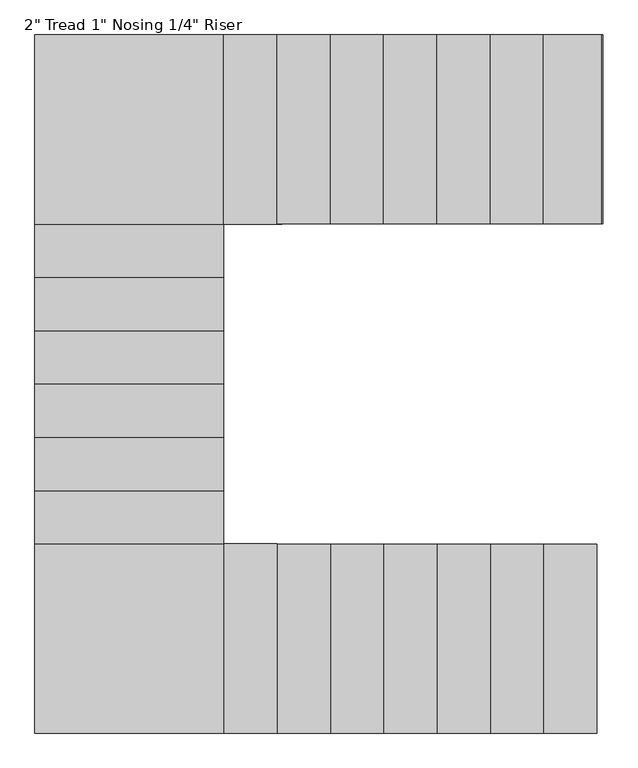
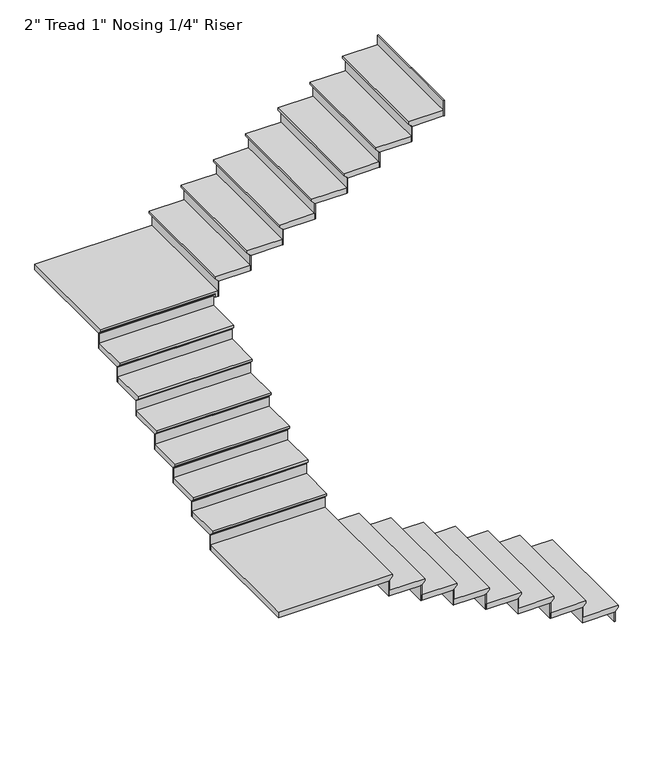
"""IFC4 building model written with IfcOpenShell, lengths in millimetres: stair flight geometry."""

from ifc_helpers import new_model, si_unit, origin, place, context, project, spatial, faceted_brep, source, transform, mapped, element, save


def stair_flight_046a0556(model_context):
    return source(origin(), model_context, "Body", "Brep", [
        faceted_brep([(-1428.1308482, -127.8399287, 119.4954545), (-1428.1308482, -127.8399287, 138.5454545), (-1428.1308482, -1118.4399287, 138.5454545), (-1428.1308482, -1118.4399287, 119.4954545), (-1453.5308482, -127.8399287, 94.0954545), (-1453.5308482, -1118.4399287, 94.0954545), (-1732.9308482, -127.8399287, 138.5454545), (-1732.9308482, -1118.4399287, 138.5454545), (-1453.5308482, -1118.4399287, 87.7454545), (-1732.9308482, -1118.4399287, 87.7454545), (-1732.9308482, -127.8399287, 87.7454545), (-1453.5308482, -127.8399287, 87.7454545)], [[[0, 1, 2, 3]], [[4, 0, 3, 5]], [[2, 1, 6, 7]], [[8, 9, 10, 11]], [[2, 7, 9, 8, 5, 3]], [[8, 11, 4, 5]], [[6, 1, 0, 4, 11, 10]], [[7, 6, 10, 9]]]),
        faceted_brep([(-1453.5308482, -127.8399287, 87.7454545), (-1453.5308482, -127.8399287, 0.0), (-1459.8808482, -127.8399287, 0.0), (-1459.8808482, -127.8399287, 87.7454545), (-1453.5308482, -1118.4399287, 87.7454545), (-1459.8808482, -1118.4399287, 87.7454545), (-1459.8808482, -1118.4399287, 0.0), (-1453.5308482, -1118.4399287, 0.0)], [[[0, 1, 2, 3]], [[4, 5, 6, 7]], [[1, 0, 4, 7]], [[2, 1, 7, 6]], [[3, 2, 6, 5]], [[0, 3, 5, 4]]]),
        faceted_brep([(-1732.9308482, -127.8399287, 226.2909091), (-1732.9308482, -127.8399287, 87.7454545), (-1739.2808482, -127.8399287, 87.7454545), (-1739.2808482, -127.8399287, 226.2909091), (-1732.9308482, -1118.4399287, 226.2909091), (-1739.2808482, -1118.4399287, 226.2909091), (-1739.2808482, -1118.4399287, 87.7454545), (-1732.9308482, -1118.4399287, 87.7454545)], [[[0, 1, 2, 3]], [[4, 5, 6, 7]], [[1, 0, 4, 7]], [[2, 1, 7, 6]], [[3, 2, 6, 5]], [[0, 3, 5, 4]]]),
        faceted_brep([(-1707.5308482, -1118.4399287, 277.0909091), (-1707.5308482, -127.8399287, 277.0909091), (-2012.3308482, -127.8399287, 277.0909091), (-2012.3308482, -1118.4399287, 277.0909091), (-1732.9308482, -1118.4399287, 226.2909091), (-2012.3308482, -1118.4399287, 226.2909091), (-2012.3308482, -127.8399287, 226.2909091), (-1732.9308482, -127.8399287, 226.2909091), (-1732.9308482, -1118.4399287, 232.6409091), (-1707.5308482, -1118.4399287, 258.0409091), (-1732.9308482, -127.8399287, 232.6409091), (-1707.5308482, -127.8399287, 258.0409091)], [[[0, 1, 2, 3]], [[4, 5, 6, 7]], [[0, 3, 5, 4, 8, 9]], [[4, 7, 10, 8]], [[2, 1, 11, 10, 7, 6]], [[3, 2, 6, 5]], [[11, 1, 0, 9]], [[10, 11, 9, 8]]]),
        faceted_brep([(-2012.3308482, -127.8399287, 364.8363636), (-2012.3308482, -127.8399287, 226.2909091), (-2018.6808482, -127.8399287, 226.2909091), (-2018.6808482, -127.8399287, 364.8363636), (-2012.3308482, -1118.4399287, 364.8363636), (-2018.6808482, -1118.4399287, 364.8363636), (-2018.6808482, -1118.4399287, 226.2909091), (-2012.3308482, -1118.4399287, 226.2909091)], [[[0, 1, 2, 3]], [[4, 5, 6, 7]], [[1, 0, 4, 7]], [[2, 1, 7, 6]], [[3, 2, 6, 5]], [[0, 3, 5, 4]]]),
        faceted_brep([(-1986.9308482, -1118.4399287, 415.6363636), (-1986.9308482, -127.8399287, 415.6363636), (-2291.7308482, -127.8399287, 415.6363636), (-2291.7308482, -1118.4399287, 415.6363636), (-2012.3308482, -1118.4399287, 364.8363636), (-2291.7308482, -1118.4399287, 364.8363636), (-2291.7308482, -127.8399287, 364.8363636), (-2012.3308482, -127.8399287, 364.8363636), (-2012.3308482, -1118.4399287, 371.1863636), (-1986.9308482, -1118.4399287, 396.5863636), (-2012.3308482, -127.8399287, 371.1863636), (-1986.9308482, -127.8399287, 396.5863636)], [[[0, 1, 2, 3]], [[4, 5, 6, 7]], [[0, 3, 5, 4, 8, 9]], [[4, 7, 10, 8]], [[2, 1, 11, 10, 7, 6]], [[3, 2, 6, 5]], [[11, 1, 0, 9]], [[10, 11, 9, 8]]]),
        faceted_brep([(-2291.7308482, -127.8399287, 503.3818182), (-2291.7308482, -127.8399287, 364.8363636), (-2298.0808482, -127.8399287, 364.8363636), (-2298.0808482, -127.8399287, 503.3818182), (-2291.7308482, -1118.4399287, 503.3818182), (-2298.0808482, -1118.4399287, 503.3818182), (-2298.0808482, -1118.4399287, 364.8363636), (-2291.7308482, -1118.4399287, 364.8363636)], [[[0, 1, 2, 3]], [[4, 5, 6, 7]], [[1, 0, 4, 7]], [[2, 1, 7, 6]], [[3, 2, 6, 5]], [[0, 3, 5, 4]]]),
        faceted_brep([(-2266.3308482, -1118.4399287, 554.1818182), (-2266.3308482, -127.8399287, 554.1818182), (-2571.1308482, -127.8399287, 554.1818182), (-2571.1308482, -1118.4399287, 554.1818182), (-2291.7308482, -1118.4399287, 503.3818182), (-2571.1308482, -1118.4399287, 503.3818182), (-2571.1308482, -127.8399287, 503.3818182), (-2291.7308482, -127.8399287, 503.3818182), (-2291.7308482, -1118.4399287, 509.7318182), (-2266.3308482, -1118.4399287, 535.1318182), (-2291.7308482, -127.8399287, 509.7318182), (-2266.3308482, -127.8399287, 535.1318182)], [[[0, 1, 2, 3]], [[4, 5, 6, 7]], [[0, 3, 5, 4, 8, 9]], [[4, 7, 10, 8]], [[2, 1, 11, 10, 7, 6]], [[3, 2, 6, 5]], [[11, 1, 0, 9]], [[10, 11, 9, 8]]]),
        faceted_brep([(-2571.1308482, -127.8399287, 641.9272727), (-2571.1308482, -127.8399287, 503.3818182), (-2577.4808482, -127.8399287, 503.3818182), (-2577.4808482, -127.8399287, 641.9272727), (-2571.1308482, -1118.4399287, 641.9272727), (-2577.4808482, -1118.4399287, 641.9272727), (-2577.4808482, -1118.4399287, 503.3818182), (-2571.1308482, -1118.4399287, 503.3818182)], [[[0, 1, 2, 3]], [[4, 5, 6, 7]], [[1, 0, 4, 7]], [[2, 1, 7, 6]], [[3, 2, 6, 5]], [[0, 3, 5, 4]]]),
        faceted_brep([(-2545.7308482, -1118.4399287, 692.7272727), (-2545.7308482, -127.8399287, 692.7272727), (-2850.5308482, -127.8399287, 692.7272727), (-2850.5308482, -1118.4399287, 692.7272727), (-2571.1308482, -1118.4399287, 641.9272727), (-2850.5308482, -1118.4399287, 641.9272727), (-2850.5308482, -127.8399287, 641.9272727), (-2571.1308482, -127.8399287, 641.9272727), (-2571.1308482, -1118.4399287, 648.2772727), (-2545.7308482, -1118.4399287, 673.6772727), (-2571.1308482, -127.8399287, 648.2772727), (-2545.7308482, -127.8399287, 673.6772727)], [[[0, 1, 2, 3]], [[4, 5, 6, 7]], [[0, 3, 5, 4, 8, 9]], [[4, 7, 10, 8]], [[2, 1, 11, 10, 7, 6]], [[3, 2, 6, 5]], [[11, 1, 0, 9]], [[10, 11, 9, 8]]]),
        faceted_brep([(-2850.5308482, -127.8399287, 780.4727273), (-2850.5308482, -127.8399287, 641.9272727), (-2856.8808482, -127.8399287, 641.9272727), (-2856.8808482, -127.8399287, 780.4727273), (-2850.5308482, -1118.4399287, 780.4727273), (-2856.8808482, -1118.4399287, 780.4727273), (-2856.8808482, -1118.4399287, 641.9272727), (-2850.5308482, -1118.4399287, 641.9272727)], [[[0, 1, 2, 3]], [[4, 5, 6, 7]], [[1, 0, 4, 7]], [[2, 1, 7, 6]], [[3, 2, 6, 5]], [[0, 3, 5, 4]]]),
        faceted_brep([(-2825.1308482, -1118.4399287, 831.2727273), (-2825.1308482, -127.8399287, 831.2727273), (-3129.9308482, -127.8399287, 831.2727273), (-3129.9308482, -1118.4399287, 831.2727273), (-2850.5308482, -1118.4399287, 780.4727273), (-3129.9308482, -1118.4399287, 780.4727273), (-3129.9308482, -127.8399287, 780.4727273), (-2850.5308482, -127.8399287, 780.4727273), (-2850.5308482, -1118.4399287, 786.8227273), (-2825.1308482, -1118.4399287, 812.2227273), (-2850.5308482, -127.8399287, 786.8227273), (-2825.1308482, -127.8399287, 812.2227273)], [[[0, 1, 2, 3]], [[4, 5, 6, 7]], [[0, 3, 5, 4, 8, 9]], [[4, 7, 10, 8]], [[2, 1, 11, 10, 7, 6]], [[3, 2, 6, 5]], [[11, 1, 0, 9]], [[10, 11, 9, 8]]]),
        faceted_brep([(-3129.9308482, -127.8399287, 919.0181818), (-3129.9308482, -127.8399287, 780.4727273), (-3136.2808482, -127.8399287, 780.4727273), (-3136.2808482, -127.8399287, 919.0181818), (-3129.9308482, -1118.4399287, 919.0181818), (-3136.2808482, -1118.4399287, 919.0181818), (-3136.2808482, -1118.4399287, 780.4727273), (-3129.9308482, -1118.4399287, 780.4727273)], [[[0, 1, 2, 3]], [[4, 5, 6, 7]], [[1, 0, 4, 7]], [[2, 1, 7, 6]], [[3, 2, 6, 5]], [[0, 3, 5, 4]]]),
        faceted_brep([(-3104.5308482, -1118.4399287, 969.8181818), (-3104.5308482, -127.8399287, 969.8181818), (-3409.3308482, -127.8399287, 969.8181818), (-3409.3308482, -1118.4399287, 969.8181818), (-3129.9308482, -1118.4399287, 919.0181818), (-3409.3308482, -1118.4399287, 919.0181818), (-3409.3308482, -127.8399287, 919.0181818), (-3129.9308482, -127.8399287, 919.0181818), (-3129.9308482, -1118.4399287, 925.3681818), (-3104.5308482, -1118.4399287, 950.7681818), (-3129.9308482, -127.8399287, 925.3681818), (-3104.5308482, -127.8399287, 950.7681818)], [[[0, 1, 2, 3]], [[4, 5, 6, 7]], [[0, 3, 5, 4, 8, 9]], [[4, 7, 10, 8]], [[2, 1, 11, 10, 7, 6]], [[3, 2, 6, 5]], [[11, 1, 0, 9]], [[10, 11, 9, 8]]]),
        faceted_brep([(-3409.3308482, -127.8399287, 1057.5636364), (-3409.3308482, -127.8399287, 919.0181818), (-3415.6808482, -127.8399287, 919.0181818), (-3415.6808482, -127.8399287, 1057.5636364), (-3409.3308482, -1118.4399287, 1057.5636364), (-3415.6808482, -1118.4399287, 1057.5636364), (-3415.6808482, -1118.4399287, 919.0181818), (-3409.3308482, -1118.4399287, 919.0181818)], [[[0, 1, 2, 3]], [[4, 5, 6, 7]], [[1, 0, 4, 7]], [[2, 1, 7, 6]], [[3, 2, 6, 5]], [[0, 3, 5, 4]]]),
        faceted_brep([(-4374.5308482, -102.4399287, 1108.3636364), (-4374.5308482, -1118.4399287, 1108.3636364), (-3383.9308482, -1118.4399287, 1108.3636364), (-3383.9308482, -102.4399287, 1108.3636364), (-4374.5308482, -1118.4399287, 1057.5636364), (-4374.5308482, -102.4399287, 1057.5636364), (-3383.9308482, -102.4399287, 1057.5636364), (-3383.9308482, -127.8399287, 1057.5636364), (-3409.3308482, -127.8399287, 1057.5636364), (-3409.3308482, -1118.4399287, 1057.5636364), (-3409.3308482, -127.8399287, 1063.9136364), (-3409.3308482, -1118.4399287, 1063.9136364), (-3383.9308482, -1118.4399287, 1089.3136364), (-3383.9308482, -127.8399287, 1089.3136364)], [[[0, 1, 2, 3]], [[4, 5, 6, 7, 8, 9]], [[1, 0, 5, 4]], [[9, 8, 10, 11]], [[3, 2, 12, 13, 7, 6]], [[0, 3, 6, 5]], [[12, 11, 10, 13]], [[2, 1, 4, 9, 11, 12]], [[8, 7, 13, 10]]]),
        faceted_brep([(-3383.9308482, -102.4399287, 1196.1090909), (-3383.9308482, -102.4399287, 1057.5636364), (-3383.9308482, -96.0899287, 1057.5636364), (-3383.9308482, -96.0899287, 1196.1090909), (-4374.5308482, -102.4399287, 1196.1090909), (-4374.5308482, -96.0899287, 1196.1090909), (-4374.5308482, -96.0899287, 1057.5636364), (-4374.5308482, -102.4399287, 1057.5636364)], [[[0, 1, 2, 3]], [[4, 5, 6, 7]], [[1, 0, 4, 7]], [[2, 1, 7, 6]], [[3, 2, 6, 5]], [[0, 3, 5, 4]]]),
        faceted_brep([(-4374.5308482, -127.8399287, 1246.9090909), (-3383.9308482, -127.8399287, 1246.9090909), (-3383.9308482, 176.9600713, 1246.9090909), (-4374.5308482, 176.9600713, 1246.9090909), (-4374.5308482, -102.4399287, 1196.1090909), (-4374.5308482, 176.9600713, 1196.1090909), (-3383.9308482, 176.9600713, 1196.1090909), (-3383.9308482, -102.4399287, 1196.1090909), (-4374.5308482, -102.4399287, 1202.4590909), (-4374.5308482, -127.8399287, 1227.8590909), (-3383.9308482, -102.4399287, 1202.4590909), (-3383.9308482, -127.8399287, 1227.8590909)], [[[0, 1, 2, 3]], [[4, 5, 6, 7]], [[0, 3, 5, 4, 8, 9]], [[4, 7, 10, 8]], [[2, 1, 11, 10, 7, 6]], [[3, 2, 6, 5]], [[11, 1, 0, 9]], [[10, 11, 9, 8]]]),
        faceted_brep([(-3383.9308482, 176.9600713, 1334.6545455), (-3383.9308482, 176.9600713, 1196.1090909), (-3383.9308482, 183.3100713, 1196.1090909), (-3383.9308482, 183.3100713, 1334.6545455), (-4374.5308482, 176.9600713, 1334.6545455), (-4374.5308482, 183.3100713, 1334.6545455), (-4374.5308482, 183.3100713, 1196.1090909), (-4374.5308482, 176.9600713, 1196.1090909)], [[[0, 1, 2, 3]], [[4, 5, 6, 7]], [[1, 0, 4, 7]], [[2, 1, 7, 6]], [[3, 2, 6, 5]], [[0, 3, 5, 4]]]),
        faceted_brep([(-4374.5308482, 151.5600713, 1385.4545455), (-3383.9308482, 151.5600713, 1385.4545455), (-3383.9308482, 456.3600713, 1385.4545455), (-4374.5308482, 456.3600713, 1385.4545455), (-4374.5308482, 176.9600713, 1334.6545455), (-4374.5308482, 456.3600713, 1334.6545455), (-3383.9308482, 456.3600713, 1334.6545455), (-3383.9308482, 176.9600713, 1334.6545455), (-4374.5308482, 176.9600713, 1341.0045455), (-4374.5308482, 151.5600713, 1366.4045455), (-3383.9308482, 176.9600713, 1341.0045455), (-3383.9308482, 151.5600713, 1366.4045455)], [[[0, 1, 2, 3]], [[4, 5, 6, 7]], [[0, 3, 5, 4, 8, 9]], [[4, 7, 10, 8]], [[2, 1, 11, 10, 7, 6]], [[3, 2, 6, 5]], [[11, 1, 0, 9]], [[10, 11, 9, 8]]]),
        faceted_brep([(-3383.9308482, 456.3600713, 1473.2), (-3383.9308482, 456.3600713, 1334.6545455), (-3383.9308482, 462.7100713, 1334.6545455), (-3383.9308482, 462.7100713, 1473.2), (-4374.5308482, 456.3600713, 1473.2), (-4374.5308482, 462.7100713, 1473.2), (-4374.5308482, 462.7100713, 1334.6545455), (-4374.5308482, 456.3600713, 1334.6545455)], [[[0, 1, 2, 3]], [[4, 5, 6, 7]], [[1, 0, 4, 7]], [[2, 1, 7, 6]], [[3, 2, 6, 5]], [[0, 3, 5, 4]]]),
        faceted_brep([(-4374.5308482, 430.9600713, 1524.0), (-3383.9308482, 430.9600713, 1524.0), (-3383.9308482, 735.7600713, 1524.0), (-4374.5308482, 735.7600713, 1524.0), (-4374.5308482, 456.3600713, 1473.2), (-4374.5308482, 735.7600713, 1473.2), (-3383.9308482, 735.7600713, 1473.2), (-3383.9308482, 456.3600713, 1473.2), (-4374.5308482, 456.3600713, 1479.55), (-4374.5308482, 430.9600713, 1504.95), (-3383.9308482, 456.3600713, 1479.55), (-3383.9308482, 430.9600713, 1504.95)], [[[0, 1, 2, 3]], [[4, 5, 6, 7]], [[0, 3, 5, 4, 8, 9]], [[4, 7, 10, 8]], [[2, 1, 11, 10, 7, 6]], [[3, 2, 6, 5]], [[11, 1, 0, 9]], [[10, 11, 9, 8]]]),
        faceted_brep([(-3383.9308482, 735.7600713, 1611.7454545), (-3383.9308482, 735.7600713, 1473.2), (-3383.9308482, 742.1100713, 1473.2), (-3383.9308482, 742.1100713, 1611.7454545), (-4374.5308482, 735.7600713, 1611.7454545), (-4374.5308482, 742.1100713, 1611.7454545), (-4374.5308482, 742.1100713, 1473.2), (-4374.5308482, 735.7600713, 1473.2)], [[[0, 1, 2, 3]], [[4, 5, 6, 7]], [[1, 0, 4, 7]], [[2, 1, 7, 6]], [[3, 2, 6, 5]], [[0, 3, 5, 4]]]),
        faceted_brep([(-4374.5308482, 710.3600713, 1662.5454545), (-3383.9308482, 710.3600713, 1662.5454545), (-3383.9308482, 1015.1600713, 1662.5454545), (-4374.5308482, 1015.1600713, 1662.5454545), (-4374.5308482, 735.7600713, 1611.7454545), (-4374.5308482, 1015.1600713, 1611.7454545), (-3383.9308482, 1015.1600713, 1611.7454545), (-3383.9308482, 735.7600713, 1611.7454545), (-4374.5308482, 735.7600713, 1618.0954545), (-4374.5308482, 710.3600713, 1643.4954545), (-3383.9308482, 735.7600713, 1618.0954545), (-3383.9308482, 710.3600713, 1643.4954545)], [[[0, 1, 2, 3]], [[4, 5, 6, 7]], [[0, 3, 5, 4, 8, 9]], [[4, 7, 10, 8]], [[2, 1, 11, 10, 7, 6]], [[3, 2, 6, 5]], [[11, 1, 0, 9]], [[10, 11, 9, 8]]]),
        faceted_brep([(-3383.9308482, 1015.1600713, 1750.2909091), (-3383.9308482, 1015.1600713, 1611.7454545), (-3383.9308482, 1021.5100713, 1611.7454545), (-3383.9308482, 1021.5100713, 1750.2909091), (-4374.5308482, 1015.1600713, 1750.2909091), (-4374.5308482, 1021.5100713, 1750.2909091), (-4374.5308482, 1021.5100713, 1611.7454545), (-4374.5308482, 1015.1600713, 1611.7454545)], [[[0, 1, 2, 3]], [[4, 5, 6, 7]], [[1, 0, 4, 7]], [[2, 1, 7, 6]], [[3, 2, 6, 5]], [[0, 3, 5, 4]]]),
        faceted_brep([(-4374.5308482, 989.7600713, 1801.0909091), (-3383.9308482, 989.7600713, 1801.0909091), (-3383.9308482, 1294.5600713, 1801.0909091), (-4374.5308482, 1294.5600713, 1801.0909091), (-4374.5308482, 1015.1600713, 1750.2909091), (-4374.5308482, 1294.5600713, 1750.2909091), (-3383.9308482, 1294.5600713, 1750.2909091), (-3383.9308482, 1015.1600713, 1750.2909091), (-4374.5308482, 1015.1600713, 1756.6409091), (-4374.5308482, 989.7600713, 1782.0409091), (-3383.9308482, 1015.1600713, 1756.6409091), (-3383.9308482, 989.7600713, 1782.0409091)], [[[0, 1, 2, 3]], [[4, 5, 6, 7]], [[0, 3, 5, 4, 8, 9]], [[4, 7, 10, 8]], [[2, 1, 11, 10, 7, 6]], [[3, 2, 6, 5]], [[11, 1, 0, 9]], [[10, 11, 9, 8]]]),
        faceted_brep([(-3383.9308482, 1294.5600713, 1888.8363636), (-3383.9308482, 1294.5600713, 1750.2909091), (-3383.9308482, 1300.9100713, 1750.2909091), (-3383.9308482, 1300.9100713, 1888.8363636), (-4374.5308482, 1294.5600713, 1888.8363636), (-4374.5308482, 1300.9100713, 1888.8363636), (-4374.5308482, 1300.9100713, 1750.2909091), (-4374.5308482, 1294.5600713, 1750.2909091)], [[[0, 1, 2, 3]], [[4, 5, 6, 7]], [[1, 0, 4, 7]], [[2, 1, 7, 6]], [[3, 2, 6, 5]], [[0, 3, 5, 4]]]),
        faceted_brep([(-4374.5308482, 1269.1600713, 1939.6363636), (-3383.9308482, 1269.1600713, 1939.6363636), (-3383.9308482, 1573.9600713, 1939.6363636), (-4374.5308482, 1573.9600713, 1939.6363636), (-4374.5308482, 1294.5600713, 1888.8363636), (-4374.5308482, 1573.9600713, 1888.8363636), (-3383.9308482, 1573.9600713, 1888.8363636), (-3383.9308482, 1294.5600713, 1888.8363636), (-4374.5308482, 1294.5600713, 1895.1863636), (-4374.5308482, 1269.1600713, 1920.5863636), (-3383.9308482, 1294.5600713, 1895.1863636), (-3383.9308482, 1269.1600713, 1920.5863636)], [[[0, 1, 2, 3]], [[4, 5, 6, 7]], [[0, 3, 5, 4, 8, 9]], [[4, 7, 10, 8]], [[2, 1, 11, 10, 7, 6]], [[3, 2, 6, 5]], [[11, 1, 0, 9]], [[10, 11, 9, 8]]]),
        faceted_brep([(-3383.9308482, 1573.9600713, 2027.3818182), (-3383.9308482, 1573.9600713, 1888.8363636), (-3383.9308482, 1580.3100713, 1888.8363636), (-3383.9308482, 1580.3100713, 2027.3818182), (-4374.5308482, 1573.9600713, 2027.3818182), (-4374.5308482, 1580.3100713, 2027.3818182), (-4374.5308482, 1580.3100713, 1888.8363636), (-4374.5308482, 1573.9600713, 1888.8363636)], [[[0, 1, 2, 3]], [[4, 5, 6, 7]], [[1, 0, 4, 7]], [[2, 1, 7, 6]], [[3, 2, 6, 5]], [[0, 3, 5, 4]]]),
        faceted_brep([(-3358.5308482, 2539.1600713, 2078.1818182), (-4374.5308482, 2539.1600713, 2078.1818182), (-4374.5308482, 1548.5600713, 2078.1818182), (-3358.5308482, 1548.5600713, 2078.1818182), (-4374.5308482, 2539.1600713, 2027.3818182), (-3358.5308482, 2539.1600713, 2027.3818182), (-3358.5308482, 1548.5600713, 2027.3818182), (-3383.9308482, 1548.5600713, 2027.3818182), (-3383.9308482, 1573.9600713, 2027.3818182), (-4374.5308482, 1573.9600713, 2027.3818182), (-3383.9308482, 1573.9600713, 2033.7318182), (-4374.5308482, 1573.9600713, 2033.7318182), (-4374.5308482, 1548.5600713, 2059.1318182), (-3383.9308482, 1548.5600713, 2059.1318182)], [[[0, 1, 2, 3]], [[4, 5, 6, 7, 8, 9]], [[1, 0, 5, 4]], [[9, 8, 10, 11]], [[3, 2, 12, 13, 7, 6]], [[0, 3, 6, 5]], [[12, 11, 10, 13]], [[2, 1, 4, 9, 11, 12]], [[8, 7, 13, 10]]]),
        faceted_brep([(-3358.5308482, 1548.5600713, 2165.9272727), (-3358.5308482, 1548.5600713, 2027.3818182), (-3352.1808482, 1548.5600713, 2027.3818182), (-3352.1808482, 1548.5600713, 2165.9272727), (-3358.5308482, 2539.1600713, 2165.9272727), (-3352.1808482, 2539.1600713, 2165.9272727), (-3352.1808482, 2539.1600713, 2027.3818182), (-3358.5308482, 2539.1600713, 2027.3818182)], [[[0, 1, 2, 3]], [[4, 5, 6, 7]], [[1, 0, 4, 7]], [[2, 1, 7, 6]], [[3, 2, 6, 5]], [[0, 3, 5, 4]]]),
        faceted_brep([(-3383.9308482, 2539.1600713, 2216.7272727), (-3383.9308482, 1548.5600713, 2216.7272727), (-3079.1308482, 1548.5600713, 2216.7272727), (-3079.1308482, 2539.1600713, 2216.7272727), (-3358.5308482, 2539.1600713, 2165.9272727), (-3079.1308482, 2539.1600713, 2165.9272727), (-3079.1308482, 1548.5600713, 2165.9272727), (-3358.5308482, 1548.5600713, 2165.9272727), (-3358.5308482, 2539.1600713, 2172.2772727), (-3383.9308482, 2539.1600713, 2197.6772727), (-3358.5308482, 1548.5600713, 2172.2772727), (-3383.9308482, 1548.5600713, 2197.6772727)], [[[0, 1, 2, 3]], [[4, 5, 6, 7]], [[0, 3, 5, 4, 8, 9]], [[4, 7, 10, 8]], [[2, 1, 11, 10, 7, 6]], [[3, 2, 6, 5]], [[11, 1, 0, 9]], [[10, 11, 9, 8]]]),
        faceted_brep([(-3079.1308482, 1548.5600713, 2304.4727273), (-3079.1308482, 1548.5600713, 2165.9272727), (-3072.7808482, 1548.5600713, 2165.9272727), (-3072.7808482, 1548.5600713, 2304.4727273), (-3079.1308482, 2539.1600713, 2304.4727273), (-3072.7808482, 2539.1600713, 2304.4727273), (-3072.7808482, 2539.1600713, 2165.9272727), (-3079.1308482, 2539.1600713, 2165.9272727)], [[[0, 1, 2, 3]], [[4, 5, 6, 7]], [[1, 0, 4, 7]], [[2, 1, 7, 6]], [[3, 2, 6, 5]], [[0, 3, 5, 4]]]),
        faceted_brep([(-3104.5308482, 2539.1600713, 2355.2727273), (-3104.5308482, 1548.5600713, 2355.2727273), (-2799.7308482, 1548.5600713, 2355.2727273), (-2799.7308482, 2539.1600713, 2355.2727273), (-3079.1308482, 2539.1600713, 2304.4727273), (-2799.7308482, 2539.1600713, 2304.4727273), (-2799.7308482, 1548.5600713, 2304.4727273), (-3079.1308482, 1548.5600713, 2304.4727273), (-3079.1308482, 2539.1600713, 2310.8227273), (-3104.5308482, 2539.1600713, 2336.2227273), (-3079.1308482, 1548.5600713, 2310.8227273), (-3104.5308482, 1548.5600713, 2336.2227273)], [[[0, 1, 2, 3]], [[4, 5, 6, 7]], [[0, 3, 5, 4, 8, 9]], [[4, 7, 10, 8]], [[2, 1, 11, 10, 7, 6]], [[3, 2, 6, 5]], [[11, 1, 0, 9]], [[10, 11, 9, 8]]]),
        faceted_brep([(-2799.7308482, 1548.5600713, 2443.0181818), (-2799.7308482, 1548.5600713, 2304.4727273), (-2793.3808482, 1548.5600713, 2304.4727273), (-2793.3808482, 1548.5600713, 2443.0181818), (-2799.7308482, 2539.1600713, 2443.0181818), (-2793.3808482, 2539.1600713, 2443.0181818), (-2793.3808482, 2539.1600713, 2304.4727273), (-2799.7308482, 2539.1600713, 2304.4727273)], [[[0, 1, 2, 3]], [[4, 5, 6, 7]], [[1, 0, 4, 7]], [[2, 1, 7, 6]], [[3, 2, 6, 5]], [[0, 3, 5, 4]]]),
        faceted_brep([(-2825.1308482, 2539.1600713, 2493.8181818), (-2825.1308482, 1548.5600713, 2493.8181818), (-2520.3308482, 1548.5600713, 2493.8181818), (-2520.3308482, 2539.1600713, 2493.8181818), (-2799.7308482, 2539.1600713, 2443.0181818), (-2520.3308482, 2539.1600713, 2443.0181818), (-2520.3308482, 1548.5600713, 2443.0181818), (-2799.7308482, 1548.5600713, 2443.0181818), (-2799.7308482, 2539.1600713, 2449.3681818), (-2825.1308482, 2539.1600713, 2474.7681818), (-2799.7308482, 1548.5600713, 2449.3681818), (-2825.1308482, 1548.5600713, 2474.7681818)], [[[0, 1, 2, 3]], [[4, 5, 6, 7]], [[0, 3, 5, 4, 8, 9]], [[4, 7, 10, 8]], [[2, 1, 11, 10, 7, 6]], [[3, 2, 6, 5]], [[11, 1, 0, 9]], [[10, 11, 9, 8]]]),
        faceted_brep([(-2520.3308482, 1548.5600713, 2581.5636364), (-2520.3308482, 1548.5600713, 2443.0181818), (-2513.9808482, 1548.5600713, 2443.0181818), (-2513.9808482, 1548.5600713, 2581.5636364), (-2520.3308482, 2539.1600713, 2581.5636364), (-2513.9808482, 2539.1600713, 2581.5636364), (-2513.9808482, 2539.1600713, 2443.0181818), (-2520.3308482, 2539.1600713, 2443.0181818)], [[[0, 1, 2, 3]], [[4, 5, 6, 7]], [[1, 0, 4, 7]], [[2, 1, 7, 6]], [[3, 2, 6, 5]], [[0, 3, 5, 4]]]),
        faceted_brep([(-2545.7308482, 2539.1600713, 2632.3636364), (-2545.7308482, 1548.5600713, 2632.3636364), (-2240.9308482, 1548.5600713, 2632.3636364), (-2240.9308482, 2539.1600713, 2632.3636364), (-2520.3308482, 2539.1600713, 2581.5636364), (-2240.9308482, 2539.1600713, 2581.5636364), (-2240.9308482, 1548.5600713, 2581.5636364), (-2520.3308482, 1548.5600713, 2581.5636364), (-2520.3308482, 2539.1600713, 2587.9136364), (-2545.7308482, 2539.1600713, 2613.3136364), (-2520.3308482, 1548.5600713, 2587.9136364), (-2545.7308482, 1548.5600713, 2613.3136364)], [[[0, 1, 2, 3]], [[4, 5, 6, 7]], [[0, 3, 5, 4, 8, 9]], [[4, 7, 10, 8]], [[2, 1, 11, 10, 7, 6]], [[3, 2, 6, 5]], [[11, 1, 0, 9]], [[10, 11, 9, 8]]]),
        faceted_brep([(-2240.9308482, 1548.5600713, 2720.1090909), (-2240.9308482, 1548.5600713, 2581.5636364), (-2234.5808482, 1548.5600713, 2581.5636364), (-2234.5808482, 1548.5600713, 2720.1090909), (-2240.9308482, 2539.1600713, 2720.1090909), (-2234.5808482, 2539.1600713, 2720.1090909), (-2234.5808482, 2539.1600713, 2581.5636364), (-2240.9308482, 2539.1600713, 2581.5636364)], [[[0, 1, 2, 3]], [[4, 5, 6, 7]], [[1, 0, 4, 7]], [[2, 1, 7, 6]], [[3, 2, 6, 5]], [[0, 3, 5, 4]]]),
        faceted_brep([(-2266.3308482, 2539.1600713, 2770.9090909), (-2266.3308482, 1548.5600713, 2770.9090909), (-1961.5308482, 1548.5600713, 2770.9090909), (-1961.5308482, 2539.1600713, 2770.9090909), (-2240.9308482, 2539.1600713, 2720.1090909), (-1961.5308482, 2539.1600713, 2720.1090909), (-1961.5308482, 1548.5600713, 2720.1090909), (-2240.9308482, 1548.5600713, 2720.1090909), (-2240.9308482, 2539.1600713, 2726.4590909), (-2266.3308482, 2539.1600713, 2751.8590909), (-2240.9308482, 1548.5600713, 2726.4590909), (-2266.3308482, 1548.5600713, 2751.8590909)], [[[0, 1, 2, 3]], [[4, 5, 6, 7]], [[0, 3, 5, 4, 8, 9]], [[4, 7, 10, 8]], [[2, 1, 11, 10, 7, 6]], [[3, 2, 6, 5]], [[11, 1, 0, 9]], [[10, 11, 9, 8]]]),
        faceted_brep([(-1961.5308482, 1548.5600713, 2858.6545455), (-1961.5308482, 1548.5600713, 2720.1090909), (-1955.1808482, 1548.5600713, 2720.1090909), (-1955.1808482, 1548.5600713, 2858.6545455), (-1961.5308482, 2539.1600713, 2858.6545455), (-1955.1808482, 2539.1600713, 2858.6545455), (-1955.1808482, 2539.1600713, 2720.1090909), (-1961.5308482, 2539.1600713, 2720.1090909)], [[[0, 1, 2, 3]], [[4, 5, 6, 7]], [[1, 0, 4, 7]], [[2, 1, 7, 6]], [[3, 2, 6, 5]], [[0, 3, 5, 4]]]),
        faceted_brep([(-1986.9308482, 2539.1600713, 2909.4545455), (-1986.9308482, 1548.5600713, 2909.4545455), (-1682.1308482, 1548.5600713, 2909.4545455), (-1682.1308482, 2539.1600713, 2909.4545455), (-1961.5308482, 2539.1600713, 2858.6545455), (-1682.1308482, 2539.1600713, 2858.6545455), (-1682.1308482, 1548.5600713, 2858.6545455), (-1961.5308482, 1548.5600713, 2858.6545455), (-1961.5308482, 2539.1600713, 2865.0045455), (-1986.9308482, 2539.1600713, 2890.4045455), (-1961.5308482, 1548.5600713, 2865.0045455), (-1986.9308482, 1548.5600713, 2890.4045455)], [[[0, 1, 2, 3]], [[4, 5, 6, 7]], [[0, 3, 5, 4, 8, 9]], [[4, 7, 10, 8]], [[2, 1, 11, 10, 7, 6]], [[3, 2, 6, 5]], [[11, 1, 0, 9]], [[10, 11, 9, 8]]]),
        faceted_brep([(-1682.1308482, 1548.5600713, 2997.2), (-1682.1308482, 1548.5600713, 2858.6545455), (-1675.7808482, 1548.5600713, 2858.6545455), (-1675.7808482, 1548.5600713, 2997.2), (-1682.1308482, 2539.1600713, 2997.2), (-1675.7808482, 2539.1600713, 2997.2), (-1675.7808482, 2539.1600713, 2858.6545455), (-1682.1308482, 2539.1600713, 2858.6545455)], [[[0, 1, 2, 3]], [[4, 5, 6, 7]], [[1, 0, 4, 7]], [[2, 1, 7, 6]], [[3, 2, 6, 5]], [[0, 3, 5, 4]]]),
        faceted_brep([(-1402.7308482, 1548.5600713, 3135.7454545), (-1402.7308482, 1548.5600713, 2997.2), (-1396.3808482, 1548.5600713, 2997.2), (-1396.3808482, 1548.5600713, 3135.7454545), (-1402.7308482, 2539.1600713, 3135.7454545), (-1396.3808482, 2539.1600713, 3135.7454545), (-1396.3808482, 2539.1600713, 2997.2), (-1402.7308482, 2539.1600713, 2997.2)], [[[0, 1, 2, 3]], [[4, 5, 6, 7]], [[1, 0, 4, 7]], [[2, 1, 7, 6]], [[3, 2, 6, 5]], [[0, 3, 5, 4]]]),
        faceted_brep([(-1707.5308482, 2539.1600713, 3048.0), (-1707.5308482, 1548.5600713, 3048.0), (-1402.7308482, 1548.5600713, 3048.0), (-1402.7308482, 2539.1600713, 3048.0), (-1682.1308482, 2539.1600713, 2997.2), (-1402.7308482, 2539.1600713, 2997.2), (-1402.7308482, 1548.5600713, 2997.2), (-1682.1308482, 1548.5600713, 2997.2), (-1682.1308482, 2539.1600713, 3003.55), (-1707.5308482, 2539.1600713, 3028.95), (-1682.1308482, 1548.5600713, 3003.55), (-1707.5308482, 1548.5600713, 3028.95)], [[[0, 1, 2, 3]], [[4, 5, 6, 7]], [[0, 3, 5, 4, 8, 9]], [[4, 7, 10, 8]], [[2, 1, 11, 10, 7, 6]], [[3, 2, 6, 5]], [[11, 1, 0, 9]], [[10, 11, 9, 8]]]),
    ])


if __name__ == "__main__":
    model = new_model("IFC4")
    model_context = context("Model", 3, world=origin())
    ifc_project = project(units=[si_unit("LENGTHUNIT", "METRE", prefix="MILLI")], contexts=[model_context])
    site = spatial("IfcSite", under=ifc_project)
    building = spatial("IfcBuilding", under=site)
    placement = place(None, origin())
    stair_flight_shape = stair_flight_046a0556(model_context)
    element("IfcStairFlight", 1, ObjectType="2\" Tread 1\" Nosing 1/4\" Riser", at=placement, inside=building, context=model_context, shape_type="MappedRepresentation", body=[
        mapped(stair_flight_shape, transform((0.0, 0.0, 0.0), x_axis=(1.0, 0.0, 0.0), y_axis=(0.0, 1.0, 0.0), z_axis=(0.0, 0.0, 1.0))),
    ])
    save(model, "model.ifc")
